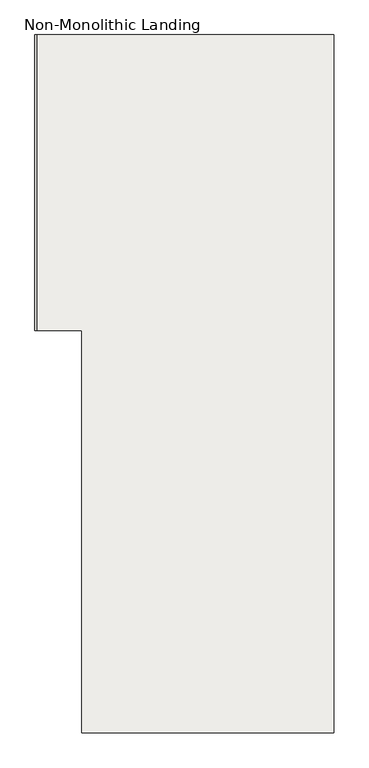
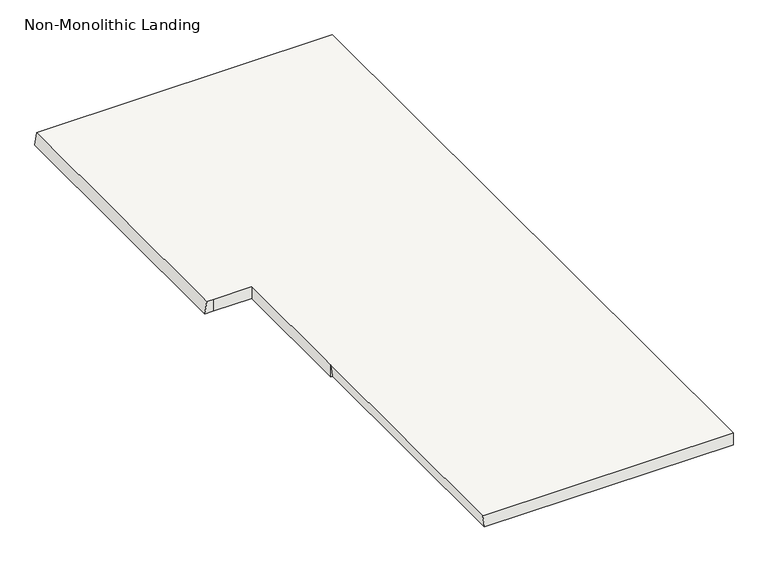
"""IFC4 building model written with IfcOpenShell, lengths in millimetres: slab geometry, Non-Monolithic Landing."""

from ifc_helpers import new_model, si_unit, origin, place, context, project, spatial, faceted_brep, source, transform, mapped, element, save


def non_monolithic_landing_709e637c(model_context):
    return source(origin(), model_context, "Body", "Brep", [
        faceted_brep([(667.2052675, 5845.1517528, 1217.3913043), (660.0177675, 5845.1517528, 1167.3913043), (660.0177675, 4668.9227481, 1167.3913043), (667.2052675, 4668.9227481, 1217.3913043), (846.727323, 3071.4281795, 1217.3913043), (1846.7531043, 3071.4281795, 1217.3913043), (1846.7531043, 5845.1517528, 1217.3913043), (692.2052675, 5845.1517528, 1217.3913043), (692.2052675, 4668.9227481, 1217.3913043), (846.727323, 4668.9227481, 1217.3913043), (846.727323, 4121.4539608, 1217.3913043), (1846.7531043, 5845.1517528, 1167.3913043), (1846.7531043, 3071.4281795, 1167.3913043), (853.914823, 3071.4281795, 1167.3913043), (853.914823, 4121.4539608, 1167.3913043), (846.727323, 4121.4539608, 1167.3913043), (846.727323, 4668.9227481, 1167.3913043), (692.2052675, 4668.9227481, 1167.3913043), (692.2052675, 5845.1517528, 1167.3913043)], [[[0, 1, 2, 3]], [[4, 5, 6, 7, 0, 3, 8, 9, 10]], [[11, 12, 13, 14, 15, 16, 17, 2, 1, 18]], [[5, 4, 13, 12]], [[6, 5, 12, 11]], [[7, 6, 11, 18]], [[0, 7, 18, 1]], [[8, 3, 2, 17]], [[9, 8, 17, 16]], [[10, 9, 16, 15]], [[14, 10, 15]], [[10, 14, 13, 4]]]),
    ])


if __name__ == "__main__":
    model = new_model("IFC4")
    model_context = context("Model", 3, world=origin())
    ifc_project = project(units=[si_unit("LENGTHUNIT", "METRE", prefix="MILLI")], contexts=[model_context])
    site = spatial("IfcSite", under=ifc_project)
    building = spatial("IfcBuilding", under=site)
    placement = place(None, origin())
    non_monolithic_landing_shape = non_monolithic_landing_709e637c(model_context)
    element("IfcSlab", 1, ObjectType="Non-Monolithic Landing", at=placement, inside=building, context=model_context, shape_type="MappedRepresentation", body=[
        mapped(non_monolithic_landing_shape, transform((0.0, 0.0, 0.0), x_axis=(1.0, 0.0, 0.0), y_axis=(0.0, 1.0, 0.0), z_axis=(0.0, 0.0, 1.0))),
    ])
    save(model, "model.ifc")
